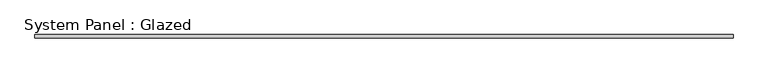
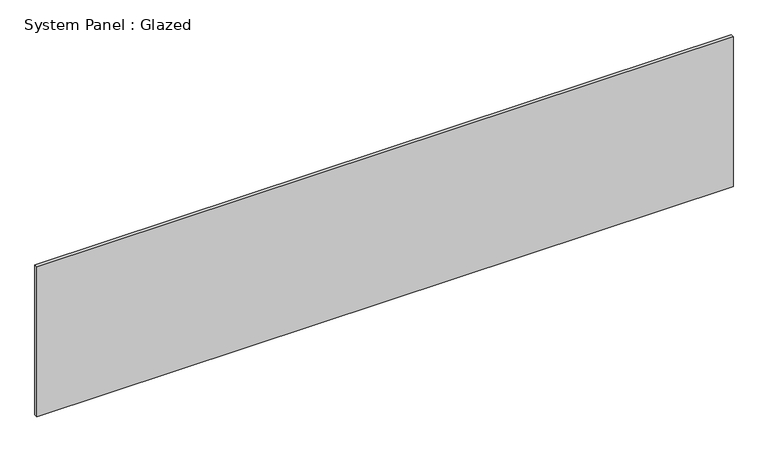
"""IFC4 building model written with IfcOpenShell, lengths in millimetres: plate geometry, System Panel : Glazed."""

from ifc_helpers import new_model, si_unit, origin, origin_with_axes, place, context, project, spatial, polyline, outline, extrude, source, transform, mapped, element, save


def system_panel_glazed_a0600ee7(model_context):
    return source(origin(), model_context, "Body", "SweptSolid", [
        extrude(outline(polyline([(2539.2990733, 19.05), (-2539.2990733, 19.05), (-2539.2990733, 44.45), (2539.2990733, 44.45), (2539.2990733, 19.05)])), origin_with_axes(), (0.0, 0.0, 1.0), 1155.7),
    ])


if __name__ == "__main__":
    model = new_model("IFC4")
    model_context = context("Model", 3, world=origin())
    ifc_project = project(units=[si_unit("LENGTHUNIT", "METRE", prefix="MILLI")], contexts=[model_context])
    site = spatial("IfcSite", under=ifc_project)
    building = spatial("IfcBuilding", under=site)
    placement = place(None, origin())
    system_panel_glazed_shape = system_panel_glazed_a0600ee7(model_context)
    element("IfcPlate", 1, ObjectType="System Panel : Glazed", at=placement, inside=building, context=model_context, shape_type="MappedRepresentation", body=[
        mapped(system_panel_glazed_shape, transform((0.0, 0.0, 0.0), x_axis=(1.0, 0.0, 0.0), y_axis=(0.0, 1.0, 0.0), z_axis=(0.0, 0.0, 1.0))),
    ])
    save(model, "model.ifc")

# Revit data of these elements
# Type "System Panel : Glazed"
#   Construction Type Id = "GSP4R"
#   Analytic Construction = "1/8 in Pilkington single glazing"
#   Visual Light Transmittance = 0.9
#   Solar Heat Gain Coefficient = 0.86
#   Heat Transfer Coefficient (U) = 1.18115 BTU/(h·ft²·°F)
# Element 1 (IfcPlate, "System Panel : Glazed")
#   Materials on its faces: "Glass"
# Materials
#   "Glass": class "Glass", colour RGB 0 128 192, transparency 0.75, Description = "Soda Lime Glass", Cost = 0
